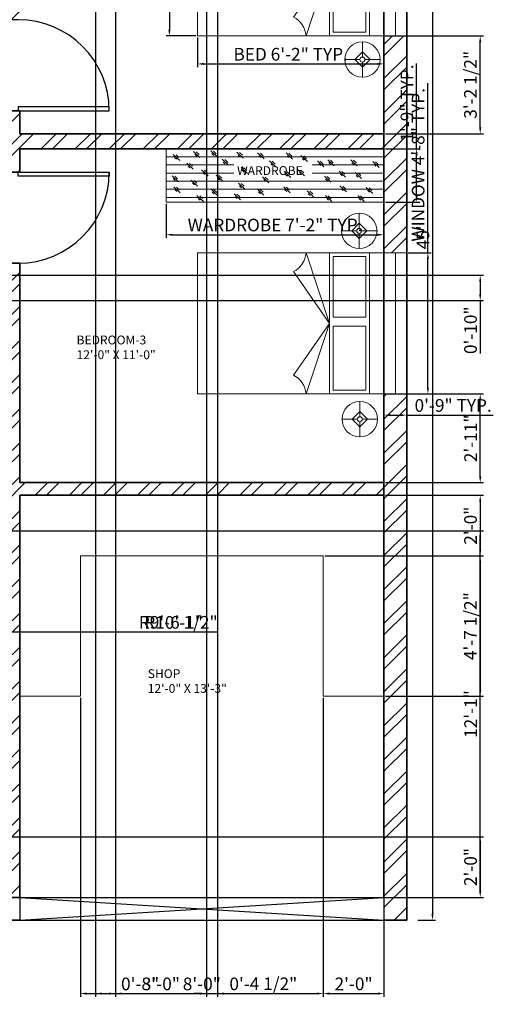
# Model space of a CAD drawing. Units: inches. Extents: x 28986 to 29505, y -162 to 451.
# Tile 4 of 6: x 29318 to 29505, y -162 to 228. Entities that reach past the tile are written whole.
import ezdxf

# ---------------------------------------------------------------- set-up
doc = ezdxf.new("R2010")
doc.units = ezdxf.units.IN
doc.layers.get('Defpoints').update_dxf_attribs({"color": 120})
for name, color, linetype, lineweight, true_color in [('A-ANNO-DIMS', 9, 'Continuous', 18, 0xafd9aa), ('A-FLOR-CASE', 32, 'Continuous', 18, 0xcd6928), ('A-FLOR-CASE-PATT', 32, 'Continuous', 13, 0xcd6928)]:
    doc.layers.add(name, color=color, linetype=linetype, lineweight=lineweight, true_color=true_color)
for name, color, linetype, lineweight in [('A-ANNO-TEXT', 6, 'Continuous', 18), ('A-AREA-IDEN', 6, 'Continuous', 18), ('A-GLAZ', 4, 'Continuous', 18), ('A-WALL', 7, 'Continuous', 35), ('A-WALL-PATT', 1, 'Continuous', 13), ('DOOR', 2, 'Continuous', 25), ('FURNITURE', 241, 'Continuous', 18)]:
    doc.layers.add(name, color=color, linetype=linetype, lineweight=lineweight)
doc.styles.get("Standard").update_dxf_attribs({"font": 'arial.ttf'})
doc.dimstyles.new('ISO-25', dxfattribs={"dimtxt": 5, "dimasz": 2.5, "dimexe": 1.25, "dimexo": 0.625, "dimtad": 1, "dimdec": 0, "dimlunit": 3, "dimtxsty": 'Standard', "dimcen": 2.5, "dimadec": 0, "dimazin": 0, "dimtfac": 1, "dimtdec": 0, "dimtmove": 0, "dimatfit": 3, "dimfxl": 1, "dimarcsym": 0})

# ---------------------------------------------------------------- blocks, each defined once
blk = doc.blocks.new('*U7')
for p, q in [((-40, 0), (-40, 6)), ((0, 0), (0, 6))]:
    blk.add_line(p, q)
blk.add_lwpolyline([(0, 0), (0, -40), (-1.75, -40), (-1.75, 0)], close=True)
blk.add_arc((0, 0), 40, 180, 270)
blk = doc.blocks.new('*U8')
for p, q in [((0, 0), (0, 6)), ((40, 0), (40, 6))]:
    blk.add_line(p, q)
blk.add_lwpolyline([(0, 0), (0, -40), (1.75, -40), (1.75, 0)], close=True)
blk.add_arc((0, 0), 40, 270, 0)
blk = doc.blocks.new('modern bed')
for p, q in [((-55.85, 73.76), (-55.85, 0)), ((0, 0), (0, 73.76)), ((-55.85, 68.07), (0, 68.07)), ((-54.35, 66.57), (-54.35, 53.68)), ((-54.35, 66.57), (-30.33, 66.57)), ((-30.33, 66.57), (-30.33, 53.68)), ((-26.87, 66.57), (-1.5, 66.57)), ((-26.87, 66.57), (-26.87, 53.68)), ((-1.5, 53.68), (-1.5, 66.57)), ((-55.85, 52.18), (0, 52.18)), ((-27.93, 52.18), (-55.85, 42.95)), ((-54.35, 53.68), (-30.33, 53.68)), ((-27.93, 52.18), (-48.41, 38.03)), ((-27.93, 52.18), (0, 42.95)), ((-27.93, 52.18), (-7.44, 38.03)), ((-26.87, 53.68), (-1.5, 53.68)), ((-55.85, 0), (0, 0))]:
    blk.add_line(p, q)
blk.add_lwpolyline([(-55.85, 73.76), (0, 73.76)])
for centre, start, end in [((-56.5, 33.89), 27.0819, 85.9278), ((0.64, 33.89), 94.0722, 152.9181)]:
    blk.add_arc(centre, 9.08, start, end)
blk = doc.blocks.new('Lamp - Table')
for p, q in [((0, 7), (0, 1)), ((-1, 0), (-7, 0)), ((0, 3), (-3, 0)), ((-3, 0), (0, -3)), ((3, 0), (0, 3)), ((0, -3), (3, 0)), ((1, 0), (7, 0)), ((0, -1), (0, -7))]:
    blk.add_line(p, q)
for radius in [7, 1]:
    blk.add_circle((0, 0), radius)
blk = doc.blocks.new('*D26')
at = {"layer": 'A-ANNO-DIMS', "color": 0, "lineweight": -2, "transparency": 16777216}
for p, q in [((29475.53, 411.7), (29482.59, 411.7)), ((29481.34, 409.2), (29481.34, -125.8)), ((29475.53, -128.3), (29482.59, -128.3))]:
    blk.add_line(p, q, dxfattribs=at)
at = {"layer": 'A-ANNO-DIMS', "color": 0, "transparency": 16777216}
for points in [[(29480.93, 409.2), (29481.76, 409.2), (29481.34, 411.7)], [(29480.93, -125.8), (29481.76, -125.8), (29481.34, -128.3)]]:
    blk.add_solid(points, dxfattribs=at)
at = {"layer": 'Defpoints', "color": 0, "transparency": 16777216}
for p in [(29474.91, 411.7), (29474.91, -128.3), (29481.34, -128.3)]:
    blk.add_point(p, dxfattribs=at)
at = {"layer": 'A-ANNO-DIMS', "color": 0, "transparency": 16777216, "insert": (29478.18, 141.7), "char_height": 5, "attachment_point": 5, "rotation": 90}
blk.add_mtext("45'", dxfattribs=at)
blk = doc.blocks.new('WIN-55_85IN')
for p, q in [((0, 55.85), (9, 55.85)), ((4.5, 0), (4.5, 55.85)), ((0, 0), (9, 0))]:
    blk.add_line(p, q)
blk = doc.blocks.new('WARDROBE-86IN')
for p, q in [((10.82, 19.98), (13.37, 17.6)), ((11.91, 19.85), (13.04, 18.77)), ((17.6, 20.32), (20.15, 17.94)), ((18.69, 20.18), (19.82, 19.11)), ((27.93, 19.75), (30.48, 17.37)), ((29.03, 19.61), (30.15, 18.53)), ((2.83, 18.79), (5.37, 16.41)), ((3.32, 17.66), (4.06, 16.95)), ((3.92, 18.65), (5.05, 17.57)), ((11.31, 18.86), (12.06, 18.15)), ((18.09, 19.2), (18.84, 18.49)), ((22.1, 16.94), (24.65, 14.56)), ((22.59, 15.82), (23.34, 15.1)), ((23.2, 16.8), (24.32, 15.72)), ((28.42, 18.62), (29.17, 17.91)), ((36.16, 19.46), (38.7, 17.08)), ((36.65, 18.33), (37.39, 17.62)), ((37.25, 19.32), (38.38, 18.24)), ((40.87, 16.28), (43.41, 13.9)), ((41.96, 16.14), (43.09, 15.06)), ((47.4, 19.42), (49.95, 17.04)), ((47.89, 18.3), (48.64, 17.59)), ((48.5, 19.29), (49.62, 18.21)), ((53.27, 18.39), (55.81, 16.01)), ((53.76, 17.27), (54.5, 16.55)), ((54.36, 18.25), (55.49, 17.17)), ((59.84, 16.27), (62.39, 13.89)), ((60.94, 16.13), (62.06, 15.05)), ((63.85, 16.72), (66.39, 14.34)), ((64.34, 15.6), (65.08, 14.88)), ((64.94, 16.58), (66.07, 15.5)), ((72.96, 16.7), (75.51, 14.32)), ((74.06, 16.56), (75.18, 15.48)), ((81.71, 16.01), (84.25, 13.63)), ((82.8, 15.87), (83.93, 14.79)), ((8.19, 15.38), (10.73, 13)), ((8.68, 14.26), (9.42, 13.54)), ((9.28, 15.24), (10.41, 14.16)), ((14, 12.81), (16.55, 10.43)), ((14.49, 11.68), (15.24, 10.97)), ((15.1, 12.67), (16.22, 11.59)), ((29.63, 13.72), (32.17, 11.34)), ((30.11, 12.59), (30.86, 11.88)), ((30.72, 13.58), (31.85, 12.5)), ((41.36, 15.15), (42.1, 14.44)), ((46.7, 12.07), (49.24, 9.69)), ((47.79, 11.93), (48.92, 10.85)), ((52.19, 12.81), (54.74, 10.43)), ((52.68, 11.68), (53.43, 10.97)), ((53.29, 12.67), (54.41, 11.59)), ((60.33, 15.14), (61.08, 14.43)), ((68.4, 12.2), (70.94, 9.82)), ((69.49, 12.07), (70.62, 10.99)), ((73.45, 15.57), (74.2, 14.86)), ((82.2, 14.88), (82.95, 14.17)), ((2.31, 10.42), (4.85, 8.04)), ((2.79, 9.29), (3.54, 8.58)), ((3.4, 10.28), (4.53, 9.2)), ((9.91, 8.72), (12.45, 6.34)), ((11, 8.58), (12.13, 7.5)), ((19.79, 10.66), (22.34, 8.28)), ((20.28, 9.54), (21.03, 8.82)), ((20.88, 10.52), (22.01, 9.44)), ((38.06, 10.04), (40.6, 7.66)), ((38.55, 8.92), (39.29, 8.2)), ((39.15, 9.9), (40.28, 8.82)), ((47.19, 10.94), (47.93, 10.23)), ((62.53, 10.24), (65.07, 7.86)), ((63.02, 9.12), (63.76, 8.4)), ((63.62, 10.1), (64.75, 9.02)), ((68.89, 11.08), (69.63, 10.37)), ((74.68, 11.68), (77.23, 9.3)), ((75.17, 10.55), (75.92, 9.84)), ((75.77, 11.54), (76.9, 10.46)), ((3.05, 6.03), (5.59, 3.65)), ((3.54, 4.91), (4.28, 4.2)), ((4.14, 5.89), (5.27, 4.82)), ((10.4, 7.6), (11.15, 6.88)), ((17.77, 5.05), (20.31, 2.67)), ((18.25, 3.92), (19, 3.21)), ((18.86, 4.91), (19.99, 3.83)), ((28.55, 7.52), (31.1, 5.14)), ((29.04, 6.4), (29.79, 5.68)), ((29.65, 7.38), (30.77, 6.3)), ((36.07, 5.13), (38.62, 2.75)), ((36.56, 4), (37.31, 3.29)), ((37.17, 4.99), (38.29, 3.91)), ((46.49, 6.03), (49.03, 3.65)), ((46.97, 4.9), (47.72, 4.19)), ((47.58, 5.89), (48.71, 4.81)), ((55.71, 4.42), (58.25, 2.04)), ((56.8, 4.28), (57.93, 3.2)), ((68.68, 6.41), (71.23, 4.03)), ((69.17, 5.28), (69.92, 4.57)), ((69.78, 6.27), (70.9, 5.19)), ((79.11, 5.8), (81.65, 3.42)), ((79.6, 4.67), (80.34, 3.96)), ((80.2, 5.66), (81.33, 4.58)), ((12.18, 2.6), (14.73, 0.22)), ((12.67, 1.47), (13.42, 0.76)), ((13.28, 2.46), (14.4, 1.38)), ((26.9, 3.3), (29.44, 0.92)), ((27.39, 2.18), (28.13, 1.46)), ((27.99, 3.16), (29.12, 2.08)), ((56.2, 3.29), (56.94, 2.58)), ((62.98, 2.55), (65.52, 0.17)), ((63.47, 1.43), (64.21, 0.72)), ((64.07, 2.42), (65.2, 1.34)), ((75.74, 2.55), (78.28, 0.17)), ((76.23, 1.43), (76.97, 0.72)), ((76.83, 2.42), (77.96, 1.34))]:
    blk.add_line(p, q)
blk.add_lwpolyline([(86.1, 21.04), (0, 21.04), (0, 0), (86.1, 0)], close=True)
blk = doc.blocks.new('*D33')
at = {"layer": 'A-ANNO-DIMS', "color": 0, "lineweight": -2, "transparency": 16777216}
for p, q in [((29388.4, 220.75), (29388.4, 209.06)), ((29462.16, 220.75), (29462.16, 209.06)), ((29390.9, 210.31), (29459.66, 210.31))]:
    blk.add_line(p, q, dxfattribs=at)
at = {"layer": 'A-ANNO-DIMS', "color": 0, "transparency": 16777216}
for points in [[(29390.9, 210.72), (29390.9, 209.89), (29388.4, 210.31)], [(29459.66, 210.72), (29459.66, 209.89), (29462.16, 210.31)]]:
    blk.add_solid(points, dxfattribs=at)
at = {"layer": 'Defpoints', "color": 0, "transparency": 16777216}
for p in [(29388.4, 221.37), (29462.16, 221.37), (29462.16, 210.31)]:
    blk.add_point(p, dxfattribs=at)
at = {"layer": 'A-ANNO-DIMS', "color": 0, "transparency": 16777216, "insert": (29425.28, 213.49), "char_height": 5, "attachment_point": 5}
blk.add_mtext('BED 6\'-2" TYP.', dxfattribs=at)
blk = doc.blocks.new('*D34')
at = {"layer": 'A-ANNO-DIMS', "color": 0, "lineweight": -2, "transparency": 16777216}
for p, q in [((29387.77, 277.22), (29376.08, 277.22)), ((29377.33, 274.72), (29377.33, 223.87)), ((29387.77, 221.37), (29376.08, 221.37))]:
    blk.add_line(p, q, dxfattribs=at)
at = {"layer": 'A-ANNO-DIMS', "color": 0, "transparency": 16777216}
for points in [[(29376.92, 274.72), (29377.75, 274.72), (29377.33, 277.22)], [(29376.92, 223.87), (29377.75, 223.87), (29377.33, 221.37)]]:
    blk.add_solid(points, dxfattribs=at)
at = {"layer": 'Defpoints', "color": 0, "transparency": 16777216}
for p in [(29388.4, 277.22), (29377.33, 221.37), (29388.4, 221.37)]:
    blk.add_point(p, dxfattribs=at)
at = {"layer": 'A-ANNO-DIMS', "color": 0, "transparency": 16777216, "insert": (29374.15, 249.3), "char_height": 5, "attachment_point": 5, "rotation": 90}
blk.add_mtext('4\'-8" TYP.', dxfattribs=at)
blk = doc.blocks.new('*D43')
at = {"layer": 'A-ANNO-DIMS', "color": 0, "lineweight": -2, "transparency": 16777216}
for p, q in [((29479.53, 135.64), (29479.53, 202.66)), ((29471.78, 135.64), (29480.78, 135.64)), ((29479.53, 82.28), (29479.53, 133.14)), ((29471.78, 79.78), (29480.78, 79.78))]:
    blk.add_line(p, q, dxfattribs=at)
at = {"layer": 'A-ANNO-DIMS', "color": 0, "transparency": 16777216}
for points in [[(29479.12, 133.14), (29479.95, 133.14), (29479.53, 135.64)], [(29479.12, 82.28), (29479.95, 82.28), (29479.53, 79.78)]]:
    blk.add_solid(points, dxfattribs=at)
at = {"layer": 'Defpoints', "color": 0, "transparency": 16777216}
for p in [(29471.16, 135.64), (29479.53, 135.64), (29471.16, 79.78)]:
    blk.add_point(p, dxfattribs=at)
at = {"layer": 'A-ANNO-DIMS', "color": 0, "transparency": 16777216, "insert": (29476.32, 170.4), "char_height": 5, "attachment_point": 5, "rotation": 90}
blk.add_mtext('WINDOW 4\'-8" TYP.', dxfattribs=at)
blk = doc.blocks.new('*D44')
at = {"layer": 'A-ANNO-DIMS', "color": 0, "lineweight": -2, "transparency": 16777216}
for p, q in [((29462.16, 79.16), (29462.16, 70.16)), ((29471.16, 79.16), (29471.16, 70.16)), ((29464.66, 71.41), (29468.66, 71.41)), ((29471.16, 71.41), (29505.38, 71.41))]:
    blk.add_line(p, q, dxfattribs=at)
at = {"layer": 'A-ANNO-DIMS', "color": 0, "transparency": 16777216}
for points in [[(29464.66, 71.82), (29464.66, 70.99), (29462.16, 71.41)], [(29468.66, 71.82), (29468.66, 70.99), (29471.16, 71.41)]]:
    blk.add_solid(points, dxfattribs=at)
at = {"layer": 'Defpoints', "color": 0, "transparency": 16777216}
for p in [(29462.16, 79.78), (29471.16, 79.78), (29471.16, 71.41)]:
    blk.add_point(p, dxfattribs=at)
at = {"layer": 'A-ANNO-DIMS', "color": 0, "transparency": 16777216, "insert": (29489.52, 74.59), "char_height": 5, "attachment_point": 5}
blk.add_mtext('0\'-9" TYP.', dxfattribs=at)
blk = doc.blocks.new('*D45')
at = {"layer": 'A-ANNO-DIMS', "color": 0, "lineweight": -2, "transparency": 16777216}
for p, q in [((29376.06, 155.03), (29376.06, 141.49)), ((29462.16, 155.03), (29462.16, 141.49)), ((29378.56, 142.74), (29459.66, 142.74))]:
    blk.add_line(p, q, dxfattribs=at)
at = {"layer": 'A-ANNO-DIMS', "color": 0, "transparency": 16777216}
for points in [[(29378.56, 143.16), (29378.56, 142.33), (29376.06, 142.74)], [(29459.66, 143.16), (29459.66, 142.33), (29462.16, 142.74)]]:
    blk.add_solid(points, dxfattribs=at)
at = {"layer": 'Defpoints', "color": 0, "transparency": 16777216}
for p in [(29376.06, 155.66), (29462.16, 155.66), (29462.16, 142.74)]:
    blk.add_point(p, dxfattribs=at)
at = {"layer": 'A-ANNO-DIMS', "color": 0, "transparency": 16777216, "insert": (29419.11, 145.95), "char_height": 5, "attachment_point": 5}
blk.add_mtext('WARDROBE 7\'-2" TYP.', dxfattribs=at)
blk = doc.blocks.new('*D46')
at = {"layer": 'A-ANNO-DIMS', "color": 0, "lineweight": -2, "transparency": 16777216}
for p, q in [((29475.07, 176.7), (29475.07, 210.46)), ((29462.78, 176.7), (29476.32, 176.7)), ((29475.07, 158.16), (29475.07, 174.2)), ((29462.78, 155.66), (29476.32, 155.66))]:
    blk.add_line(p, q, dxfattribs=at)
at = {"layer": 'A-ANNO-DIMS', "color": 0, "transparency": 16777216}
for points in [[(29474.65, 174.2), (29475.49, 174.2), (29475.07, 176.7)], [(29474.65, 158.16), (29475.49, 158.16), (29475.07, 155.66)]]:
    blk.add_solid(points, dxfattribs=at)
at = {"layer": 'Defpoints', "color": 0, "transparency": 16777216}
for p in [(29462.16, 176.7), (29475.07, 176.7), (29462.16, 155.66)]:
    blk.add_point(p, dxfattribs=at)
at = {"layer": 'A-ANNO-DIMS', "color": 0, "transparency": 16777216, "insert": (29471.89, 194.83), "char_height": 5, "attachment_point": 5, "rotation": 90}
blk.add_mtext('1\'-9" TYP.', dxfattribs=at)
blk = doc.blocks.new('*D65')
at = {"layer": 'A-ANNO-DIMS', "color": 0, "lineweight": -2, "transparency": 16777216}
for p, q in [((29168.78, 25.7), (29501.46, 25.7)), ((29500.21, -116.8), (29500.21, 23.2)), ((29168.78, -119.3), (29501.46, -119.3))]:
    blk.add_line(p, q, dxfattribs=at)
at = {"layer": 'A-ANNO-DIMS', "color": 0, "transparency": 16777216}
for points in [[(29499.79, 23.2), (29500.62, 23.2), (29500.21, 25.7)], [(29499.79, -116.8), (29500.62, -116.8), (29500.21, -119.3)]]:
    blk.add_solid(points, dxfattribs=at)
at = {"layer": 'Defpoints', "color": 0, "transparency": 16777216}
for p in [(29168.16, 25.7), (29500.21, 25.7), (29168.16, -119.3)]:
    blk.add_point(p, dxfattribs=at)
at = {"layer": 'A-ANNO-DIMS', "color": 0, "transparency": 16777216, "insert": (29497.07, -46.8), "char_height": 5, "attachment_point": 5, "rotation": 90}
blk.add_mtext('12\'-1"', dxfattribs=at)
blk = doc.blocks.new('*D68')
at = {"layer": 'A-ANNO-DIMS', "color": 0, "lineweight": -2, "transparency": 16777216}
for p, q in [((29462.78, 221.37), (29501.46, 221.37)), ((29500.21, 185.2), (29500.21, 218.87)), ((29462.78, 182.7), (29501.46, 182.7))]:
    blk.add_line(p, q, dxfattribs=at)
at = {"layer": 'A-ANNO-DIMS', "color": 0, "transparency": 16777216}
for points in [[(29499.79, 218.87), (29500.62, 218.87), (29500.21, 221.37)], [(29499.79, 185.2), (29500.62, 185.2), (29500.21, 182.7)]]:
    blk.add_solid(points, dxfattribs=at)
at = {"layer": 'Defpoints', "color": 0, "transparency": 16777216}
for p in [(29462.16, 221.37), (29500.21, 221.37), (29462.16, 182.7)]:
    blk.add_point(p, dxfattribs=at)
at = {"layer": 'A-ANNO-DIMS', "color": 0, "transparency": 16777216, "insert": (29496.99, 202.04), "char_height": 5, "attachment_point": 5, "rotation": 90}
blk.add_mtext('3\'-2 1/2"', dxfattribs=at)
blk = doc.blocks.new('*D69')
at = {"layer": 'A-ANNO-DIMS', "color": 0, "lineweight": -2, "transparency": 16777216}
for p, q in [((29462.78, 79.78), (29501.46, 79.78)), ((29500.21, 47.2), (29500.21, 77.28)), ((29462.78, 44.7), (29501.46, 44.7))]:
    blk.add_line(p, q, dxfattribs=at)
at = {"layer": 'A-ANNO-DIMS', "color": 0, "transparency": 16777216}
for points in [[(29499.79, 77.28), (29500.62, 77.28), (29500.21, 79.78)], [(29499.79, 47.2), (29500.62, 47.2), (29500.21, 44.7)]]:
    blk.add_solid(points, dxfattribs=at)
at = {"layer": 'Defpoints', "color": 0, "transparency": 16777216}
for p in [(29462.16, 79.78), (29500.21, 79.78), (29462.16, 44.7)]:
    blk.add_point(p, dxfattribs=at)
at = {"layer": 'A-ANNO-DIMS', "color": 0, "transparency": 16777216, "insert": (29497.07, 62.24), "char_height": 5, "attachment_point": 5, "rotation": 90}
blk.add_mtext('2\'-11"', dxfattribs=at)
blk = doc.blocks.new('*D79')
at = {"layer": 'A-ANNO-DIMS', "color": 0, "lineweight": -2, "transparency": 16777216}
for p, q in [((29355.99, 326.07), (29355.99, -158.6)), ((29391.99, 326.07), (29391.99, -158.6)), ((29358.49, -157.35), (29389.49, -157.35))]:
    blk.add_line(p, q, dxfattribs=at)
at = {"layer": 'A-ANNO-DIMS', "color": 0, "transparency": 16777216}
for points in [[(29358.49, -156.93), (29358.49, -157.77), (29355.99, -157.35)], [(29389.49, -156.93), (29389.49, -157.77), (29391.99, -157.35)]]:
    blk.add_solid(points, dxfattribs=at)
at = {"layer": 'Defpoints', "color": 0, "transparency": 16777216}
for p in [(29355.99, 326.7), (29391.99, 326.7), (29391.99, -157.35)]:
    blk.add_point(p, dxfattribs=at)
at = {"layer": 'A-ANNO-DIMS', "color": 0, "transparency": 16777216, "insert": (29373.99, -154.17), "char_height": 5, "attachment_point": 5}
blk.add_mtext('3\'-0"', dxfattribs=at)
blk = doc.blocks.new('*D80')
at = {"layer": 'A-ANNO-DIMS', "color": 0, "lineweight": -2, "transparency": 16777216}
for p, q in [((29348.16, 332.07), (29348.16, -158.6)), ((29355.99, 332.07), (29355.99, -158.6)), ((29350.66, -157.35), (29353.49, -157.35)), ((29355.99, -157.35), (29373.03, -157.35))]:
    blk.add_line(p, q, dxfattribs=at)
at = {"layer": 'A-ANNO-DIMS', "color": 0, "transparency": 16777216}
for points in [[(29350.66, -156.93), (29350.66, -157.77), (29348.16, -157.35)], [(29353.49, -156.93), (29353.49, -157.77), (29355.99, -157.35)]]:
    blk.add_solid(points, dxfattribs=at)
at = {"layer": 'Defpoints', "color": 0, "transparency": 16777216}
for p in [(29348.16, 332.7), (29355.99, 332.7), (29355.99, -157.35)]:
    blk.add_point(p, dxfattribs=at)
at = {"layer": 'A-ANNO-DIMS', "color": 0, "transparency": 16777216, "insert": (29365.76, -154.17), "char_height": 5, "attachment_point": 5}
blk.add_mtext('0\'-8"', dxfattribs=at)
blk = doc.blocks.new('*D89')
at = {"layer": 'A-ANNO-DIMS', "color": 0, "lineweight": -2, "transparency": 16777216}
for p, q in [((29084.78, -95.3), (29501.46, -95.3)), ((29500.21, -97.8), (29500.21, -116.8)), ((29084.78, -119.3), (29501.46, -119.3))]:
    blk.add_line(p, q, dxfattribs=at)
at = {"layer": 'A-ANNO-DIMS', "color": 0, "transparency": 16777216}
for points in [[(29499.79, -97.8), (29500.62, -97.8), (29500.21, -95.3)], [(29499.79, -116.8), (29500.62, -116.8), (29500.21, -119.3)]]:
    blk.add_solid(points, dxfattribs=at)
at = {"layer": 'Defpoints', "color": 0, "transparency": 16777216}
for p in [(29084.16, -95.3), (29084.16, -119.3), (29500.21, -119.3)]:
    blk.add_point(p, dxfattribs=at)
at = {"layer": 'A-ANNO-DIMS', "color": 0, "transparency": 16777216, "insert": (29497.03, -107.3), "char_height": 5, "attachment_point": 5, "rotation": 90}
blk.add_mtext('2\'-0"', dxfattribs=at)
blk = doc.blocks.new('*D91')
at = {"layer": 'A-ANNO-DIMS', "color": 0, "lineweight": -2, "transparency": 16777216}
for p, q in [((29096.78, 126.7), (29501.46, 126.7)), ((29500.21, 124.2), (29500.21, 119.2)), ((29096.78, 116.7), (29501.46, 116.7)), ((29500.21, 116.7), (29500.21, 95.77))]:
    blk.add_line(p, q, dxfattribs=at)
at = {"layer": 'A-ANNO-DIMS', "color": 0, "transparency": 16777216}
for points in [[(29499.79, 124.2), (29500.62, 124.2), (29500.21, 126.7)], [(29499.79, 119.2), (29500.62, 119.2), (29500.21, 116.7)]]:
    blk.add_solid(points, dxfattribs=at)
at = {"layer": 'Defpoints', "color": 0, "transparency": 16777216}
for p in [(29096.16, 126.7), (29096.16, 116.7), (29500.21, 116.7)]:
    blk.add_point(p, dxfattribs=at)
at = {"layer": 'A-ANNO-DIMS', "color": 0, "transparency": 16777216, "insert": (29497.03, 104.99), "char_height": 5, "attachment_point": 5, "rotation": 90}
blk.add_mtext('0\'-10"', dxfattribs=at)
blk = doc.blocks.new('*D92')
at = {"layer": 'A-ANNO-DIMS', "color": 0, "lineweight": -2, "transparency": 16777216}
for p, q in [((29342.16, -40.43), (29342.16, -158.6)), ((29438.16, -40.43), (29438.16, -158.6)), ((29344.66, -157.35), (29435.66, -157.35))]:
    blk.add_line(p, q, dxfattribs=at)
at = {"layer": 'A-ANNO-DIMS', "color": 0, "transparency": 16777216}
for points in [[(29344.66, -156.93), (29344.66, -157.77), (29342.16, -157.35)], [(29435.66, -156.93), (29435.66, -157.77), (29438.16, -157.35)]]:
    blk.add_solid(points, dxfattribs=at)
at = {"layer": 'Defpoints', "color": 0, "transparency": 16777216}
for p in [(29342.16, -39.8), (29438.16, -39.8), (29438.16, -157.35)]:
    blk.add_point(p, dxfattribs=at)
at = {"layer": 'A-ANNO-DIMS', "color": 0, "transparency": 16777216, "insert": (29390.16, -154.17), "char_height": 5, "attachment_point": 5}
blk.add_mtext('8\'-0"', dxfattribs=at)
blk = doc.blocks.new('*D93')
at = {"layer": 'A-ANNO-DIMS', "color": 0, "lineweight": -2, "transparency": 16777216}
for p, q in [((29438.16, -40.43), (29438.16, -158.6)), ((29462.16, -40.43), (29462.16, -158.6)), ((29440.66, -157.35), (29459.66, -157.35))]:
    blk.add_line(p, q, dxfattribs=at)
at = {"layer": 'A-ANNO-DIMS', "color": 0, "transparency": 16777216}
for points in [[(29440.66, -156.93), (29440.66, -157.77), (29438.16, -157.35)], [(29459.66, -156.93), (29459.66, -157.77), (29462.16, -157.35)]]:
    blk.add_solid(points, dxfattribs=at)
at = {"layer": 'Defpoints', "color": 0, "transparency": 16777216}
for p in [(29438.16, -39.8), (29462.16, -39.8), (29462.16, -157.35)]:
    blk.add_point(p, dxfattribs=at)
at = {"layer": 'A-ANNO-DIMS', "color": 0, "transparency": 16777216, "insert": (29450.16, -154.17), "char_height": 5, "attachment_point": 5}
blk.add_mtext('2\'-0"', dxfattribs=at)
blk = doc.blocks.new('*D94')
at = {"layer": 'A-ANNO-DIMS', "color": 0, "lineweight": -2, "transparency": 16777216}
for p, q in [((29462.78, 39.7), (29501.46, 39.7)), ((29500.21, 37.2), (29500.21, 18.2)), ((29438.78, 15.7), (29501.46, 15.7))]:
    blk.add_line(p, q, dxfattribs=at)
at = {"layer": 'A-ANNO-DIMS', "color": 0, "transparency": 16777216}
for points in [[(29499.79, 37.2), (29500.62, 37.2), (29500.21, 39.7)], [(29499.79, 18.2), (29500.62, 18.2), (29500.21, 15.7)]]:
    blk.add_solid(points, dxfattribs=at)
at = {"layer": 'Defpoints', "color": 0, "transparency": 16777216}
for p in [(29462.16, 39.7), (29438.16, 15.7), (29500.21, 15.7)]:
    blk.add_point(p, dxfattribs=at)
at = {"layer": 'A-ANNO-DIMS', "color": 0, "transparency": 16777216, "insert": (29497.03, 27.7), "char_height": 5, "attachment_point": 5, "rotation": 90}
blk.add_mtext('2\'-0"', dxfattribs=at)
blk = doc.blocks.new('*D95')
at = {"layer": 'A-ANNO-DIMS', "color": 0, "lineweight": -2, "transparency": 16777216}
for p, q in [((29438.78, 15.7), (29501.46, 15.7)), ((29500.21, 13.2), (29500.21, -37.3)), ((29462.78, -39.8), (29501.46, -39.8))]:
    blk.add_line(p, q, dxfattribs=at)
at = {"layer": 'A-ANNO-DIMS', "color": 0, "transparency": 16777216}
for points in [[(29499.79, 13.2), (29500.62, 13.2), (29500.21, 15.7)], [(29499.79, -37.3), (29500.62, -37.3), (29500.21, -39.8)]]:
    blk.add_solid(points, dxfattribs=at)
at = {"layer": 'Defpoints', "color": 0, "transparency": 16777216}
for p in [(29438.16, 15.7), (29462.16, -39.8), (29500.21, -39.8)]:
    blk.add_point(p, dxfattribs=at)
at = {"layer": 'A-ANNO-DIMS', "color": 0, "transparency": 16777216, "insert": (29497, -12.05), "char_height": 5, "attachment_point": 5, "rotation": 90}
blk.add_mtext('4\'-7 1/2"', dxfattribs=at)
blk = doc.blocks.new('*D96')
at = {"layer": 'A-ANNO-DIMS', "color": 0, "lineweight": -2, "transparency": 16777216}
for p, q in [((29391.99, 326.07), (29391.99, -158.6)), ((29396.38, 326.07), (29396.38, -158.6)), ((29389.49, -157.35), (29386.99, -157.35)), ((29391.99, -157.35), (29396.38, -157.35)), ((29398.88, -157.35), (29427.57, -157.35))]:
    blk.add_line(p, q, dxfattribs=at)
at = {"layer": 'A-ANNO-DIMS', "color": 0, "transparency": 16777216}
for points in [[(29389.49, -156.93), (29389.49, -157.77), (29391.99, -157.35)], [(29398.88, -156.93), (29398.88, -157.77), (29396.38, -157.35)]]:
    blk.add_solid(points, dxfattribs=at)
at = {"layer": 'Defpoints', "color": 0, "transparency": 16777216}
for p in [(29391.99, 326.7), (29396.38, 326.7), (29396.38, -157.35)]:
    blk.add_point(p, dxfattribs=at)
at = {"layer": 'A-ANNO-DIMS', "color": 0, "transparency": 16777216, "insert": (29414.48, -154.14), "char_height": 5, "attachment_point": 5}
blk.add_mtext('0\'-4 1/2"', dxfattribs=at)
blk = doc.blocks.new('*D99')
at = {"layer": 'A-ANNO-DIMS', "color": 0, "lineweight": -2, "transparency": 16777216}
for p, q in [((29185.1, -14.39), (29306.29, -14.39)), ((29390.62, -14.39), (29308.79, -14.39))]:
    blk.add_line(p, q, dxfattribs=at)
at = {"layer": 'A-ANNO-DIMS', "color": 0, "transparency": 16777216}
blk.add_solid([(29308.79, -13.98), (29308.79, -14.81), (29306.29, -14.39)], dxfattribs=at)
at = {"layer": 'Defpoints', "color": 0, "transparency": 16777216}
for p in [(29185.1, -14.39), (29306.29, -14.39)]:
    blk.add_point(p, dxfattribs=at)
at = {"layer": 'A-ANNO-DIMS', "color": 0, "transparency": 16777216, "insert": (29379.01, -11.22), "char_height": 5, "attachment_point": 5, "rotation": 0}
blk.add_mtext('R10\'-1"', dxfattribs=at)
blk = doc.blocks.new('*D100')
at = {"layer": 'A-ANNO-DIMS', "color": 0, "lineweight": -2, "transparency": 16777216}
for p, q in [((29198.04, -14.39), (29312.29, -14.39)), ((29396.33, -14.39), (29314.79, -14.39))]:
    blk.add_line(p, q, dxfattribs=at)
at = {"layer": 'A-ANNO-DIMS', "color": 0, "transparency": 16777216}
blk.add_solid([(29314.79, -13.98), (29314.79, -14.81), (29312.29, -14.39)], dxfattribs=at)
at = {"layer": 'Defpoints', "color": 0, "transparency": 16777216}
for p in [(29198.04, -14.39), (29312.29, -14.39)]:
    blk.add_point(p, dxfattribs=at)
at = {"layer": 'A-ANNO-DIMS', "color": 0, "transparency": 16777216, "insert": (29380.84, -11.18), "char_height": 5, "attachment_point": 5, "rotation": 0}
blk.add_mtext('R9\'-6 1/2"', dxfattribs=at)

msp = doc.modelspace()

# ---------------------------------------------------------------- hatches: boundary and pattern name
at = {"layer": 'A-WALL-PATT'}
h = msp.add_hatch(dxfattribs=at)
h.set_pattern_fill('ANSI32', color=256)
h.paths.add_polyline_path([(29174.16, 34.7), (29163.04, 34.7), (29163.04, 29.3), (29163.04, 25.7), (29168.16, 25.7), (29168.16, -119.3), (29174.16, -119.3), (29174.16, -71.3), (29199.96, -71.3), (29199.96, -65.3), (29174.16, -65.3)])
h.paths.add_polyline_path([(29244.8, -65.3), (29235.96, -65.3), (29235.96, -71.3), (29244.8, -71.3)])
h.paths.add_polyline_path([(29318.16, 39.7), (29462.16, 39.7), (29462.16, 44.7), (29318.16, 44.7), (29318.16, 131.49), (29312.16, 131.49), (29312.16, -65.3), (29292.8, -65.3), (29292.8, -71.3), (29312.16, -71.3), (29312.16, -119.3), (29318.16, -119.3)])
h.paths.add_polyline_path([(29219.6, 411.7), (29051.16, 411.7), (29051.16, 368.84), (29060.16, 368.84), (29060.16, 402.7), (29204.16, 402.7), (29219.6, 402.7)])
h.paths.add_polyline_path([(29060.16, 320.84), (29051.16, 320.84), (29051.16, 231.24), (29060.16, 231.24), (29060.16, 252.7)])
h.paths.add_polyline_path([(29210.16, 265.69), (29204.76, 265.69), (29204.16, 265.69), (29204.16, 258.7), (29060.16, 258.7), (29060.16, 252.7), (29204.16, 252.7), (29204.16, 228.7), (29204.16, 168.7), (29199.96, 168.7), (29199.96, 167.47), (29199.96, 162.7), (29210.16, 162.7)])
h.paths.add_polyline_path([(29060.16, 183.24), (29051.16, 183.24), (29051.16, 162.7), (29060.16, 162.7), (29168.16, 162.7), (29168.16, 167.47), (29168.16, 168.7), (29060.16, 168.7)])
h.paths.add_polyline_path([(29060.16, 126.7), (29051.16, 126.7), (29051.16, 70.7), (29060.16, 70.7)])
h.paths.add_polyline_path([(29060.16, 25.7), (29127.04, 25.7), (29127.04, 34.7), (29060.16, 34.7), (29051.16, 34.7), (29051.16, -22.45), (29060.16, -22.45)])
h.paths.add_polyline_path([(29060.16, -70.45), (29051.16, -70.45), (29051.16, -128.3), (29084.16, -128.3), (29084.16, -119.3), (29060.16, -119.3)])
h.paths.add_polyline_path([(29174.16, -119.3), (29168.16, -119.3), (29132.16, -119.3), (29132.16, -128.3), (29174.16, -128.3)])
h.paths.add_polyline_path([(29471.16, 79.78), (29462.16, 79.78), (29462.16, -119.3), (29462.16, -128.3), (29471.16, -128.3)])
h.paths.add_polyline_path([(29462.16, 182.7), (29318.16, 182.7), (29318.16, 191.79), (29317.56, 191.79), (29312.16, 191.79), (29312.16, 167.49), (29317.56, 167.49), (29318.16, 167.49), (29318.16, 176.7), (29462.16, 176.7)])
h.paths.add_polyline_path([(29471.16, 221.37), (29462.16, 221.37), (29462.16, 135.64), (29471.16, 135.64)])
h.paths.add_polyline_path([(29471.16, 360.33), (29462.16, 360.33), (29462.16, 277.22), (29471.16, 277.22)])
h.paths.add_polyline_path([(29471.16, 411.7), (29243.6, 411.7), (29243.6, 402.7), (29462.16, 402.7), (29462.16, 384.33), (29471.16, 384.33)])
h.paths.add_polyline_path([(29348.16, 402.7), (29342.16, 402.7), (29342.16, 332.7), (29308.66, 332.7), (29308.66, 326.7), (29312.16, 326.7), (29312.16, 227.79), (29318.16, 227.79), (29318.16, 326.7), (29355.99, 326.7), (29355.99, 332.7), (29348.16, 332.7)])
h.paths.add_polyline_path([(29210.16, 326.7), (29272.66, 326.7), (29272.66, 332.1), (29272.66, 332.7), (29210.16, 332.7), (29210.16, 402.7), (29204.16, 402.7), (29204.16, 316.6), (29204.16, 301.69), (29210.16, 301.69)])

# ---------------------------------------------------------------- linework, layer by layer
at = {"layer": 'A-FLOR-CASE'}
for p, q in [((29438.16, 15.7), (29342.16, 15.7)), ((29342.16, 15.7), (29342.16, -39.8)), ((29318.16, -39.8), (29342.16, -39.8)), ((29438.16, -39.8), (29462.16, -39.8))]:
    msp.add_line(p, q, dxfattribs=at)
msp.add_lwpolyline([(29438.16, 15.7), (29438.16, -39.8)], dxfattribs=at)
at = {"layer": 'A-WALL'}
for p, q in [((29471.16, -128.3), (29471.16, 411.7)), ((29462.16, -119.3), (29462.16, 402.7)), ((29318.16, 191.79), (29312.16, 191.79)), ((29318.16, 191.79), (29318.16, 182.7)), ((29462.16, 182.7), (29318.16, 182.7)), ((29462.16, 176.7), (29318.16, 176.7)), ((29318.16, 176.7), (29318.16, 167.49)), ((29318.16, 167.49), (29312.16, 167.49)), ((29318.16, 131.49), (29312.16, 131.49)), ((29318.16, 131.49), (29318.16, 44.7)), ((29462.16, 44.7), (29318.16, 44.7)), ((29462.16, 39.7), (29318.16, 39.7)), ((29318.16, 39.7), (29318.16, -119.3)), ((29060.16, -119.3), (29318.16, -119.3)), ((29051.16, -128.3), (29318.16, -128.3)), ((29462.16, -128.3), (29471.16, -128.3))]:
    msp.add_line(p, q, dxfattribs=at)
msp.add_lwpolyline([(29462.16, 39.7), (29462.16, -119.3)], dxfattribs=at)
at = {"layer": 'DOOR'}
for p, q in [((29318.16, -119.3), (29462.16, -128.3)), ((29318.16, -128.3), (29462.16, -119.3)), ((29318.16, -119.3), (29462.16, -119.3)), ((29318.16, -119.3), (29318.16, -128.3)), ((29462.16, -119.3), (29462.16, -128.3)), ((29318.16, -128.3), (29462.16, -128.3))]:
    msp.add_line(p, q, dxfattribs=at)

# ---------------------------------------------------------------- block references
at = {"layer": 'A-GLAZ'}
for p in [(29462.16, 221.37), (29462.16, 79.78)]:
    msp.add_blockref('WIN-55_85IN', p, dxfattribs=at)
at = {"layer": 'DOOR', "xscale": 0.8999999999999752, "yscale": 0.8999999999999752, "zscale": 0.8999999999999752, "rotation": 90}
for name, p in [('*U8', (29317.56, 191.79)), ('*U7', (29317.56, 167.49))]:
    msp.add_blockref(name, p, dxfattribs=at)
at = {"layer": 'FURNITURE', "rotation": 270}
for p in [(29388.4, 221.37), (29388.4, 79.78)]:
    msp.add_blockref('modern bed', p, dxfattribs=at)
at = {"layer": 'FURNITURE'}
for p in [(29453.65, 212.02), (29452.41, 144.28), (29452.61, 69.8)]:
    msp.add_blockref('Lamp - Table', p, dxfattribs=at)

# ---------------------------------------------------------------- texts
at = {"layer": 'A-AREA-IDEN', "char_height": 3.5, "attachment_point": 1}
for s, insert in [('BEDROOM-3\\P12\'-0" X 11\'-0"', (29340.64, 102.88)), ('SHOP\\P12\'-0" X 13\'-3"', (29368.78, -29.09))]:
    msp.add_mtext_dynamic_manual_height_columns(s, width=65.867, gutter_width=12.5, heights=[0], dxfattribs=dict(at, insert=insert))

# ---------------------------------------------------------------- dimensions: what is measured, and where the dimension line sits
at = {"layer": 'A-ANNO-DIMS'}
for base, p1, p2, override, picture, middle in [((29481.34, -128.3), (29474.91, 411.7), (29474.91, -128.3), {"dimclrd": 0, "dimclre": 0, "dimclrt": 0}, '*D26', (29478.18, 141.7)), ((29500.21, 221.37), (29462.16, 182.7), (29462.16, 221.37), {"dimdec": 1, "dimlfac": 1, "dimrnd": 0, "dimzin": 1, "dimdsep": 46, "dimlunit": 4, "dimfrac": 2}, '*D68', (29496.99, 202.04)), ((29500.21, 116.7), (29096.16, 126.7), (29096.16, 116.7), {"dimdec": 1, "dimlfac": 1, "dimrnd": 0, "dimzin": 1, "dimdsep": 46, "dimlunit": 4, "dimfrac": 2}, '*D91', (29497.03, 104.99)), ((29500.21, 79.78), (29462.16, 44.7), (29462.16, 79.78), {"dimdec": 1, "dimlfac": 1, "dimrnd": 0, "dimzin": 1, "dimdsep": 46, "dimlunit": 4, "dimfrac": 2}, '*D69', (29497.07, 62.24)), ((29500.21, 15.7), (29462.16, 39.7), (29438.16, 15.7), {"dimdec": 1, "dimlfac": 1, "dimrnd": 0, "dimzin": 1, "dimdsep": 46, "dimlunit": 4, "dimfrac": 2}, '*D94', (29497.03, 27.7)), ((29500.21, 25.7), (29168.16, -119.3), (29168.16, 25.7), {"dimdec": 1, "dimlfac": 1, "dimrnd": 0, "dimzin": 1, "dimdsep": 46, "dimlunit": 4, "dimfrac": 2}, '*D65', (29497.07, -46.8)), ((29500.21, -39.8), (29438.16, 15.7), (29462.16, -39.8), {"dimdec": 1, "dimlfac": 1, "dimrnd": 0, "dimzin": 1, "dimdsep": 46, "dimlunit": 4, "dimfrac": 2}, '*D95', (29497, -12.05)), ((29500.21, -119.3), (29084.16, -95.3), (29084.16, -119.3), {"dimdec": 1, "dimlfac": 1, "dimrnd": 0, "dimzin": 1, "dimdsep": 46, "dimlunit": 4, "dimfrac": 2}, '*D89', (29497.03, -107.3))]:
    dim = msp.add_linear_dim(base=base, p1=p1, p2=p2, angle=90, dimstyle='ISO-25', override=override, dxfattribs=at)
    dim.commit()
    dim.dimension.update_dxf_attribs({"geometry": picture, "text_midpoint": middle})
for base, p1, p2, picture, middle in [((29355.99, -157.35), (29348.16, 332.7), (29355.99, 332.7), '*D80', (29365.76, -154.17)), ((29391.99, -157.35), (29355.99, 326.7), (29391.99, 326.7), '*D79', (29373.99, -154.17)), ((29438.16, -157.35), (29342.16, -39.8), (29438.16, -39.8), '*D92', (29390.16, -154.17)), ((29462.16, -157.35), (29438.16, -39.8), (29462.16, -39.8), '*D93', (29450.16, -154.17))]:
    dim = msp.add_linear_dim(base=base, p1=p1, p2=p2, dimstyle='ISO-25', override={"dimdec": 1, "dimlfac": 1, "dimrnd": 0, "dimzin": 1, "dimdsep": 46, "dimlunit": 4, "dimfrac": 2}, dxfattribs=at)
    dim.commit()
    dim.dimension.update_dxf_attribs({"geometry": picture, "text_midpoint": middle})
for base, p1, p2, angle, text, picture, middle in [((29377.3318, 221.3714), (29388.396, 277.2231), (29388.396, 221.3714), 270, '<> TYP.', '*D34', (29374.154, 249.2972)), ((29475.07, 176.7), (29462.16, 155.66), (29462.16, 176.7), 90, '<> TYP.', '*D46', (29471.89, 194.83)), ((29479.53, 135.64), (29471.16, 79.78), (29471.16, 135.64), 90, 'WINDOW <> TYP.', '*D43', (29476.32, 170.4))]:
    dim = msp.add_linear_dim(base=base, p1=p1, p2=p2, angle=angle, text=text, dimstyle='ISO-25', override={"dimdec": 1, "dimlfac": 1, "dimrnd": 0, "dimzin": 1, "dimdsep": 46, "dimlunit": 4, "dimfrac": 2}, dxfattribs=at)
    dim.commit()
    dim.dimension.update_dxf_attribs({"geometry": picture, "text_midpoint": middle})
for base, p1, p2, text, picture, middle in [((29462.16, 210.31), (29388.4, 221.37), (29462.16, 221.37), 'BED <> TYP.', '*D33', (29425.28, 213.49)), ((29462.16, 142.74), (29376.06, 155.66), (29462.16, 155.66), 'WARDROBE <> TYP.', '*D45', (29419.11, 145.95)), ((29471.16, 71.41), (29462.16, 79.78), (29471.16, 79.78), '<> TYP.', '*D44', (29489.52, 74.59))]:
    dim = msp.add_linear_dim(base=base, p1=p1, p2=p2, text=text, dimstyle='ISO-25', override={"dimdec": 1, "dimlfac": 1, "dimrnd": 0, "dimzin": 1, "dimdsep": 46, "dimlunit": 4, "dimfrac": 2}, dxfattribs=at)
    dim.commit()
    dim.dimension.update_dxf_attribs({"geometry": picture, "text_midpoint": middle})
for center, mpoint, picture, middle in [((29198.044791, -14.394047), (29312.294791, -14.394), '*D100', (29380.844791, -14.3939718)), ((29185.1, -14.39), (29306.29, -14.39), '*D99', (29379.01, -14.39))]:
    dim = msp.add_radius_dim(center=center, mpoint=mpoint, dimstyle='ISO-25', override={"dimdec": 1, "dimlfac": 1, "dimrnd": 0, "dimzin": 1, "dimdsep": 46, "dimlunit": 4, "dimfrac": 2}, dxfattribs=at)
    dim.commit()
    dim.dimension.update_dxf_attribs({"geometry": picture, "text_midpoint": middle, "dimtype": 164})

# ---------------------------------------------------------------- next in the draw order: wipeouts: each hides what was drawn before it
msp.add_wipeout([(29402.87, 165.01), (29433.8, 165.01), (29433.8, 171.09), (29402.87, 171.09)]).dxf.layer = 'A-ANNO-TEXT'

# ---------------------------------------------------------------- next in the draw order: hatches: boundary and pattern name
at = {"layer": 'A-FLOR-CASE-PATT'}
h = msp.add_hatch(dxfattribs=at)
h.set_pattern_fill('ANSI31', color=256, scale=1.012456, angle=-45, style=0)
h.paths.add_polyline_path([(29376.06, 155.66), (29462.16, 155.66), (29462.16, 176.7), (29376.06, 176.7)])
h.paths.add_polyline_path([(29402.87, 165.01), (29433.8, 165.01), (29433.8, 171.09), (29402.87, 171.09)], flags=0)

# ---------------------------------------------------------------- next in the draw order: block references
at = {"layer": 'A-FLOR-CASE'}
msp.add_blockref('WARDROBE-86IN', (29376.06, 155.66), dxfattribs=at)

# ---------------------------------------------------------------- next in the draw order: texts
at = {"layer": 'A-ANNO-TEXT', "insert": (29404.1, 169.86), "char_height": 3.5, "width": 65.867, "attachment_point": 1}
msp.add_mtext('WARDROBE', dxfattribs=at)

# ---------------------------------------------------------------- next in the draw order: dimensions: what is measured, and where the dimension line sits
at = {"layer": 'A-ANNO-DIMS'}
dim = msp.add_linear_dim(base=(29396.38, -157.35), p1=(29391.99, 326.7), p2=(29396.38, 326.7), dimstyle='ISO-25', override={"dimdec": 1, "dimlfac": 1, "dimrnd": 0, "dimzin": 1, "dimdsep": 46, "dimlunit": 4, "dimfrac": 2}, dxfattribs=at)
dim.commit()
dim.dimension.update_dxf_attribs({"geometry": '*D96', "text_midpoint": (29414.48, -154.14)})

doc.saveas('drawing.dxf')
